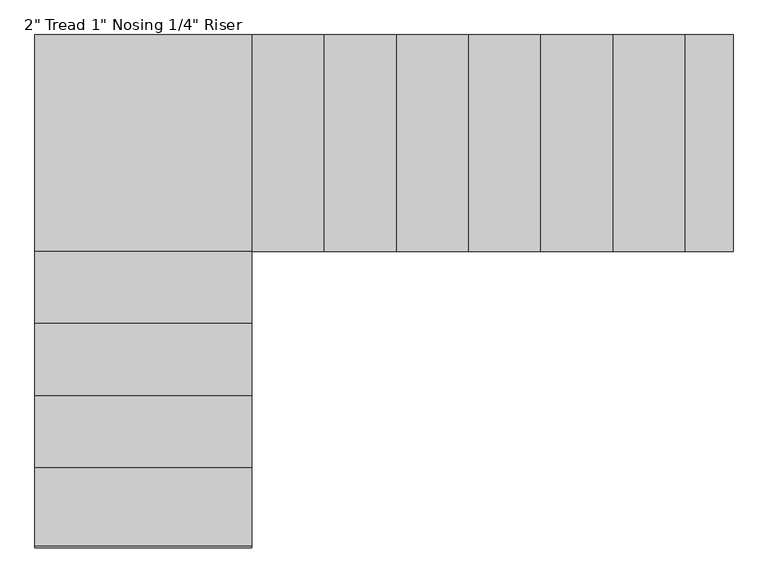
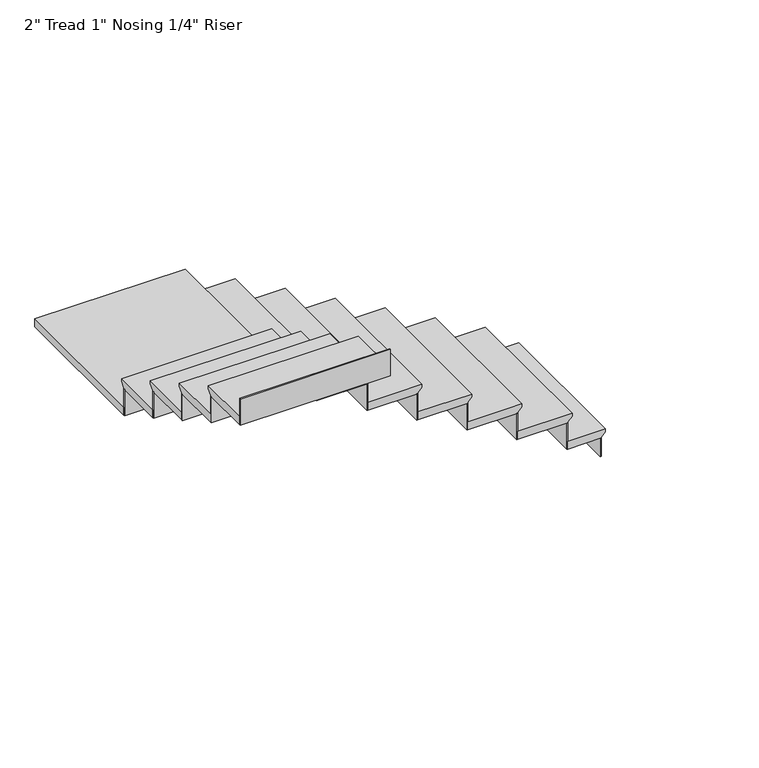
"""IFC4 building model written with IfcOpenShell, lengths in millimetres: stair flight geometry."""

from ifc_helpers import new_model, si_unit, origin, place, context, project, spatial, faceted_brep, source, transform, mapped, element, save


def stair_flight_890a58f3(model_context):
    return source(origin(), model_context, "Body", "Brep", [
        faceted_brep([(-442.4415084, 5282.3381995, 19200.2833333), (-442.4415084, 5282.3381995, 19219.3333333), (-442.4415084, 4368.3146777, 19219.3333333), (-442.4415084, 4368.3146777, 19200.2833333), (-467.8415084, 5282.3381995, 19174.8833333), (-467.8415084, 4368.3146777, 19174.8833333), (-671.0415084, 5282.3381995, 19219.3333333), (-671.0415084, 4368.3146777, 19219.3333333), (-467.8415084, 4368.3146777, 19168.5333333), (-671.0415084, 4368.3146777, 19168.5333333), (-671.0415084, 5282.3381995, 19168.5333333), (-467.8415084, 5282.3381995, 19168.5333333)], [[[0, 1, 2, 3]], [[4, 0, 3, 5]], [[2, 1, 6, 7]], [[8, 9, 10, 11]], [[2, 7, 9, 8, 5, 3]], [[8, 11, 4, 5]], [[6, 1, 0, 4, 11, 10]], [[7, 6, 10, 9]]]),
        faceted_brep([(-467.8415084, 5282.3381995, 19168.5333333), (-467.8415084, 5282.3381995, 19050.0), (-474.1915084, 5282.3381995, 19050.0), (-474.1915084, 5282.3381995, 19168.5333333), (-467.8415084, 4368.3146777, 19168.5333333), (-474.1915084, 4368.3146777, 19168.5333333), (-474.1915084, 4368.3146777, 19050.0), (-467.8415084, 4368.3146777, 19050.0)], [[[0, 1, 2, 3]], [[4, 5, 6, 7]], [[1, 0, 4, 7]], [[2, 1, 7, 6]], [[3, 2, 6, 5]], [[0, 3, 5, 4]]]),
        faceted_brep([(-671.0415084, 5282.3381995, 19337.8666667), (-671.0415084, 5282.3381995, 19168.5333333), (-677.3915084, 5282.3381995, 19168.5333333), (-677.3915084, 5282.3381995, 19337.8666667), (-671.0415084, 4368.3146777, 19337.8666667), (-677.3915084, 4368.3146777, 19337.8666667), (-677.3915084, 4368.3146777, 19168.5333333), (-671.0415084, 4368.3146777, 19168.5333333)], [[[0, 1, 2, 3]], [[4, 5, 6, 7]], [[1, 0, 4, 7]], [[2, 1, 7, 6]], [[3, 2, 6, 5]], [[0, 3, 5, 4]]]),
        faceted_brep([(-645.6415084, 4368.3146777, 19388.6666667), (-645.6415084, 5282.3381995, 19388.6666667), (-975.8415084, 5282.3381995, 19388.6666667), (-975.8415084, 4368.3146777, 19388.6666667), (-671.0415084, 4368.3146777, 19337.8666667), (-975.8415084, 4368.3146777, 19337.8666667), (-975.8415084, 5282.3381995, 19337.8666667), (-671.0415084, 5282.3381995, 19337.8666667), (-671.0415084, 4368.3146777, 19344.2166667), (-645.6415084, 4368.3146777, 19369.6166667), (-671.0415084, 5282.3381995, 19344.2166667), (-645.6415084, 5282.3381995, 19369.6166667)], [[[0, 1, 2, 3]], [[4, 5, 6, 7]], [[0, 3, 5, 4, 8, 9]], [[4, 7, 10, 8]], [[2, 1, 11, 10, 7, 6]], [[3, 2, 6, 5]], [[11, 1, 0, 9]], [[10, 11, 9, 8]]]),
        faceted_brep([(-975.8415084, 5282.3381995, 19507.2), (-975.8415084, 5282.3381995, 19337.8666667), (-982.1915084, 5282.3381995, 19337.8666667), (-982.1915084, 5282.3381995, 19507.2), (-975.8415084, 4368.3146777, 19507.2), (-982.1915084, 4368.3146777, 19507.2), (-982.1915084, 4368.3146777, 19337.8666667), (-975.8415084, 4368.3146777, 19337.8666667)], [[[0, 1, 2, 3]], [[4, 5, 6, 7]], [[1, 0, 4, 7]], [[2, 1, 7, 6]], [[3, 2, 6, 5]], [[0, 3, 5, 4]]]),
        faceted_brep([(-950.4415084, 4368.3146777, 19558.0), (-950.4415084, 5282.3381995, 19558.0), (-1280.6415084, 5282.3381995, 19558.0), (-1280.6415084, 4368.3146777, 19558.0), (-975.8415084, 4368.3146777, 19507.2), (-1280.6415084, 4368.3146777, 19507.2), (-1280.6415084, 5282.3381995, 19507.2), (-975.8415084, 5282.3381995, 19507.2), (-975.8415084, 4368.3146777, 19513.55), (-950.4415084, 4368.3146777, 19538.95), (-975.8415084, 5282.3381995, 19513.55), (-950.4415084, 5282.3381995, 19538.95)], [[[0, 1, 2, 3]], [[4, 5, 6, 7]], [[0, 3, 5, 4, 8, 9]], [[4, 7, 10, 8]], [[2, 1, 11, 10, 7, 6]], [[3, 2, 6, 5]], [[11, 1, 0, 9]], [[10, 11, 9, 8]]]),
        faceted_brep([(-1280.6415084, 5282.3381995, 19676.5333333), (-1280.6415084, 5282.3381995, 19507.2), (-1286.9915084, 5282.3381995, 19507.2), (-1286.9915084, 5282.3381995, 19676.5333333), (-1280.6415084, 4368.3146777, 19676.5333333), (-1286.9915084, 4368.3146777, 19676.5333333), (-1286.9915084, 4368.3146777, 19507.2), (-1280.6415084, 4368.3146777, 19507.2)], [[[0, 1, 2, 3]], [[4, 5, 6, 7]], [[1, 0, 4, 7]], [[2, 1, 7, 6]], [[3, 2, 6, 5]], [[0, 3, 5, 4]]]),
        faceted_brep([(-1255.2415084, 4368.3146777, 19727.3333333), (-1255.2415084, 5282.3381995, 19727.3333333), (-1585.4415084, 5282.3381995, 19727.3333333), (-1585.4415084, 4368.3146777, 19727.3333333), (-1280.6415084, 4368.3146777, 19676.5333333), (-1585.4415084, 4368.3146777, 19676.5333333), (-1585.4415084, 5282.3381995, 19676.5333333), (-1280.6415084, 5282.3381995, 19676.5333333), (-1280.6415084, 4368.3146777, 19682.8833333), (-1255.2415084, 4368.3146777, 19708.2833333), (-1280.6415084, 5282.3381995, 19682.8833333), (-1255.2415084, 5282.3381995, 19708.2833333)], [[[0, 1, 2, 3]], [[4, 5, 6, 7]], [[0, 3, 5, 4, 8, 9]], [[4, 7, 10, 8]], [[2, 1, 11, 10, 7, 6]], [[3, 2, 6, 5]], [[11, 1, 0, 9]], [[10, 11, 9, 8]]]),
        faceted_brep([(-1585.4415084, 5282.3381995, 19845.8666667), (-1585.4415084, 5282.3381995, 19676.5333333), (-1591.7915084, 5282.3381995, 19676.5333333), (-1591.7915084, 5282.3381995, 19845.8666667), (-1585.4415084, 4368.3146777, 19845.8666667), (-1591.7915084, 4368.3146777, 19845.8666667), (-1591.7915084, 4368.3146777, 19676.5333333), (-1585.4415084, 4368.3146777, 19676.5333333)], [[[0, 1, 2, 3]], [[4, 5, 6, 7]], [[1, 0, 4, 7]], [[2, 1, 7, 6]], [[3, 2, 6, 5]], [[0, 3, 5, 4]]]),
        faceted_brep([(-1560.0415084, 4368.3146777, 19896.6666667), (-1560.0415084, 5282.3381995, 19896.6666667), (-1890.2415084, 5282.3381995, 19896.6666667), (-1890.2415084, 4368.3146777, 19896.6666667), (-1585.4415084, 4368.3146777, 19845.8666667), (-1890.2415084, 4368.3146777, 19845.8666667), (-1890.2415084, 5282.3381995, 19845.8666667), (-1585.4415084, 5282.3381995, 19845.8666667), (-1585.4415084, 4368.3146777, 19852.2166667), (-1560.0415084, 4368.3146777, 19877.6166667), (-1585.4415084, 5282.3381995, 19852.2166667), (-1560.0415084, 5282.3381995, 19877.6166667)], [[[0, 1, 2, 3]], [[4, 5, 6, 7]], [[0, 3, 5, 4, 8, 9]], [[4, 7, 10, 8]], [[2, 1, 11, 10, 7, 6]], [[3, 2, 6, 5]], [[11, 1, 0, 9]], [[10, 11, 9, 8]]]),
        faceted_brep([(-1890.2415084, 5282.3381995, 20015.2), (-1890.2415084, 5282.3381995, 19845.8666667), (-1896.5915084, 5282.3381995, 19845.8666667), (-1896.5915084, 5282.3381995, 20015.2), (-1890.2415084, 4368.3146777, 20015.2), (-1896.5915084, 4368.3146777, 20015.2), (-1896.5915084, 4368.3146777, 19845.8666667), (-1890.2415084, 4368.3146777, 19845.8666667)], [[[0, 1, 2, 3]], [[4, 5, 6, 7]], [[1, 0, 4, 7]], [[2, 1, 7, 6]], [[3, 2, 6, 5]], [[0, 3, 5, 4]]]),
        faceted_brep([(-1864.8415084, 4368.3146777, 20066.0), (-1864.8415084, 5282.3381995, 20066.0), (-2195.0415084, 5282.3381995, 20066.0), (-2195.0415084, 4368.3146777, 20066.0), (-1890.2415084, 4368.3146777, 20015.2), (-2195.0415084, 4368.3146777, 20015.2), (-2195.0415084, 5282.3381995, 20015.2), (-1890.2415084, 5282.3381995, 20015.2), (-1890.2415084, 4368.3146777, 20021.55), (-1864.8415084, 4368.3146777, 20046.95), (-1890.2415084, 5282.3381995, 20021.55), (-1864.8415084, 5282.3381995, 20046.95)], [[[0, 1, 2, 3]], [[4, 5, 6, 7]], [[0, 3, 5, 4, 8, 9]], [[4, 7, 10, 8]], [[2, 1, 11, 10, 7, 6]], [[3, 2, 6, 5]], [[11, 1, 0, 9]], [[10, 11, 9, 8]]]),
        faceted_brep([(-2195.0415084, 5282.3381995, 20184.5333333), (-2195.0415084, 5282.3381995, 20015.2), (-2201.3915084, 5282.3381995, 20015.2), (-2201.3915084, 5282.3381995, 20184.5333333), (-2195.0415084, 4368.3146777, 20184.5333333), (-2201.3915084, 4368.3146777, 20184.5333333), (-2201.3915084, 4368.3146777, 20015.2), (-2195.0415084, 4368.3146777, 20015.2)], [[[0, 1, 2, 3]], [[4, 5, 6, 7]], [[1, 0, 4, 7]], [[2, 1, 7, 6]], [[3, 2, 6, 5]], [[0, 3, 5, 4]]]),
        faceted_brep([(-2169.6415084, 4368.3146777, 20235.3333333), (-2169.6415084, 5282.3381995, 20235.3333333), (-2499.8415084, 5282.3381995, 20235.3333333), (-2499.8415084, 4368.3146777, 20235.3333333), (-2195.0415084, 4368.3146777, 20184.5333333), (-2499.8415084, 4368.3146777, 20184.5333333), (-2499.8415084, 5282.3381995, 20184.5333333), (-2195.0415084, 5282.3381995, 20184.5333333), (-2195.0415084, 4368.3146777, 20190.8833333), (-2169.6415084, 4368.3146777, 20216.2833333), (-2195.0415084, 5282.3381995, 20190.8833333), (-2169.6415084, 5282.3381995, 20216.2833333)], [[[0, 1, 2, 3]], [[4, 5, 6, 7]], [[0, 3, 5, 4, 8, 9]], [[4, 7, 10, 8]], [[2, 1, 11, 10, 7, 6]], [[3, 2, 6, 5]], [[11, 1, 0, 9]], [[10, 11, 9, 8]]]),
        faceted_brep([(-2499.8415084, 5282.3381995, 20353.8666667), (-2499.8415084, 5282.3381995, 20184.5333333), (-2506.1915084, 5282.3381995, 20184.5333333), (-2506.1915084, 5282.3381995, 20353.8666667), (-2499.8415084, 4368.3146777, 20353.8666667), (-2506.1915084, 4368.3146777, 20353.8666667), (-2506.1915084, 4368.3146777, 20184.5333333), (-2499.8415084, 4368.3146777, 20184.5333333)], [[[0, 1, 2, 3]], [[4, 5, 6, 7]], [[1, 0, 4, 7]], [[2, 1, 7, 6]], [[3, 2, 6, 5]], [[0, 3, 5, 4]]]),
        faceted_brep([(-3388.8415084, 5282.3381995, 20404.6666667), (-3388.8415084, 4342.9146777, 20404.6666667), (-2474.4415084, 4342.9146777, 20404.6666667), (-2474.4415084, 5282.3381995, 20404.6666667), (-2474.4415084, 4368.3146777, 20353.8666667), (-2474.4415084, 4342.9146777, 20353.8666667), (-3388.8415084, 4342.9146777, 20353.8666667), (-3388.8415084, 5282.3381995, 20353.8666667), (-2499.8415084, 5282.3381995, 20353.8666667), (-2499.8415084, 4368.3146777, 20353.8666667), (-2474.4415084, 4368.3146777, 20385.6166667), (-2474.4415084, 5282.3381995, 20385.6166667), (-2499.8415084, 4368.3146777, 20360.2166667), (-2499.8415084, 5282.3381995, 20360.2166667)], [[[0, 1, 2, 3]], [[4, 5, 6, 7, 8, 9]], [[3, 2, 5, 4, 10, 11]], [[4, 9, 12, 10]], [[9, 8, 13, 12]], [[0, 3, 11, 13, 8, 7]], [[1, 0, 7, 6]], [[2, 1, 6, 5]], [[13, 11, 10, 12]]]),
        faceted_brep([(-3388.8415084, 4342.9146777, 20523.2), (-3388.8415084, 4342.9146777, 20353.8666667), (-3388.8415084, 4336.5646777, 20353.8666667), (-3388.8415084, 4336.5646777, 20523.2), (-2474.4415084, 4342.9146777, 20523.2), (-2474.4415084, 4336.5646777, 20523.2), (-2474.4415084, 4336.5646777, 20353.8666667), (-2474.4415084, 4342.9146777, 20353.8666667)], [[[0, 1, 2, 3]], [[4, 5, 6, 7]], [[1, 0, 4, 7]], [[2, 1, 7, 6]], [[3, 2, 6, 5]], [[0, 3, 5, 4]]]),
        faceted_brep([(-2474.4415084, 4368.3146777, 20574.0), (-3388.8415084, 4368.3146777, 20574.0), (-3388.8415084, 4037.7382512, 20574.0), (-2474.4415084, 4037.7382512, 20574.0), (-2474.4415084, 4342.9146777, 20523.2), (-2474.4415084, 4037.7382512, 20523.2), (-3388.8415084, 4037.7382512, 20523.2), (-3388.8415084, 4342.9146777, 20523.2), (-2474.4415084, 4342.9146777, 20529.55), (-2474.4415084, 4368.3146777, 20554.95), (-3388.8415084, 4342.9146777, 20529.55), (-3388.8415084, 4368.3146777, 20554.95)], [[[0, 1, 2, 3]], [[4, 5, 6, 7]], [[0, 3, 5, 4, 8, 9]], [[4, 7, 10, 8]], [[2, 1, 11, 10, 7, 6]], [[3, 2, 6, 5]], [[11, 1, 0, 9]], [[10, 11, 9, 8]]]),
        faceted_brep([(-3388.8415084, 4037.7382512, 20692.5333333), (-3388.8415084, 4037.7382512, 20523.2), (-3388.8415084, 4031.3882512, 20523.2), (-3388.8415084, 4031.3882512, 20692.5333333), (-2474.4415084, 4037.7382512, 20692.5333333), (-2474.4415084, 4031.3882512, 20692.5333333), (-2474.4415084, 4031.3882512, 20523.2), (-2474.4415084, 4037.7382512, 20523.2)], [[[0, 1, 2, 3]], [[4, 5, 6, 7]], [[1, 0, 4, 7]], [[2, 1, 7, 6]], [[3, 2, 6, 5]], [[0, 3, 5, 4]]]),
        faceted_brep([(-2474.4415084, 4063.1382512, 20743.3333333), (-3388.8415084, 4063.1382512, 20743.3333333), (-3388.8415084, 3732.938277, 20743.3333333), (-2474.4415084, 3732.938277, 20743.3333333), (-2474.4415084, 4037.7382512, 20692.5333333), (-2474.4415084, 3732.938277, 20692.5333333), (-3388.8415084, 3732.938277, 20692.5333333), (-3388.8415084, 4037.7382512, 20692.5333333), (-2474.4415084, 4037.7382512, 20698.8833333), (-2474.4415084, 4063.1382512, 20724.2833333), (-3388.8415084, 4037.7382512, 20698.8833333), (-3388.8415084, 4063.1382512, 20724.2833333)], [[[0, 1, 2, 3]], [[4, 5, 6, 7]], [[0, 3, 5, 4, 8, 9]], [[4, 7, 10, 8]], [[2, 1, 11, 10, 7, 6]], [[3, 2, 6, 5]], [[11, 1, 0, 9]], [[10, 11, 9, 8]]]),
        faceted_brep([(-3388.8415084, 3732.938277, 20861.8666667), (-3388.8415084, 3732.938277, 20692.5333333), (-3388.8415084, 3726.588277, 20692.5333333), (-3388.8415084, 3726.588277, 20861.8666667), (-2474.4415084, 3732.938277, 20861.8666667), (-2474.4415084, 3726.588277, 20861.8666667), (-2474.4415084, 3726.588277, 20692.5333333), (-2474.4415084, 3732.938277, 20692.5333333)], [[[0, 1, 2, 3]], [[4, 5, 6, 7]], [[1, 0, 4, 7]], [[2, 1, 7, 6]], [[3, 2, 6, 5]], [[0, 3, 5, 4]]]),
        faceted_brep([(-2474.4415084, 3758.338277, 20912.6666667), (-3388.8415084, 3758.338277, 20912.6666667), (-3388.8415084, 3428.1383028, 20912.6666667), (-2474.4415084, 3428.1383028, 20912.6666667), (-2474.4415084, 3732.938277, 20861.8666667), (-2474.4415084, 3428.1383028, 20861.8666667), (-3388.8415084, 3428.1383028, 20861.8666667), (-3388.8415084, 3732.938277, 20861.8666667), (-2474.4415084, 3732.938277, 20868.2166667), (-2474.4415084, 3758.338277, 20893.6166667), (-3388.8415084, 3732.938277, 20868.2166667), (-3388.8415084, 3758.338277, 20893.6166667)], [[[0, 1, 2, 3]], [[4, 5, 6, 7]], [[0, 3, 5, 4, 8, 9]], [[4, 7, 10, 8]], [[2, 1, 11, 10, 7, 6]], [[3, 2, 6, 5]], [[11, 1, 0, 9]], [[10, 11, 9, 8]]]),
        faceted_brep([(-3388.8415084, 3428.1383028, 21031.2), (-3388.8415084, 3428.1383028, 20861.8666667), (-3388.8415084, 3421.7883028, 20861.8666667), (-3388.8415084, 3421.7883028, 21031.2), (-2474.4415084, 3428.1383028, 21031.2), (-2474.4415084, 3421.7883028, 21031.2), (-2474.4415084, 3421.7883028, 20861.8666667), (-2474.4415084, 3428.1383028, 20861.8666667)], [[[0, 1, 2, 3]], [[4, 5, 6, 7]], [[1, 0, 4, 7]], [[2, 1, 7, 6]], [[3, 2, 6, 5]], [[0, 3, 5, 4]]]),
        faceted_brep([(-3388.8415084, 3123.3383287, 21200.5333333), (-3388.8415084, 3123.3383287, 21031.2), (-3388.8415084, 3116.9883287, 21031.2), (-3388.8415084, 3116.9883287, 21200.5333333), (-2474.4415084, 3123.3383287, 21200.5333333), (-2474.4415084, 3116.9883287, 21200.5333333), (-2474.4415084, 3116.9883287, 21031.2), (-2474.4415084, 3123.3383287, 21031.2)], [[[0, 1, 2, 3]], [[4, 5, 6, 7]], [[1, 0, 4, 7]], [[2, 1, 7, 6]], [[3, 2, 6, 5]], [[0, 3, 5, 4]]]),
        faceted_brep([(-2474.4415084, 3453.5383028, 21082.0), (-3388.8415084, 3453.5383028, 21082.0), (-3388.8415084, 3123.3383287, 21082.0), (-2474.4415084, 3123.3383287, 21082.0), (-2474.4415084, 3428.1383028, 21031.2), (-2474.4415084, 3123.3383287, 21031.2), (-3388.8415084, 3123.3383287, 21031.2), (-3388.8415084, 3428.1383028, 21031.2), (-2474.4415084, 3428.1383028, 21037.55), (-2474.4415084, 3453.5383028, 21062.95), (-3388.8415084, 3428.1383028, 21037.55), (-3388.8415084, 3453.5383028, 21062.95)], [[[0, 1, 2, 3]], [[4, 5, 6, 7]], [[0, 3, 5, 4, 8, 9]], [[4, 7, 10, 8]], [[2, 1, 11, 10, 7, 6]], [[3, 2, 6, 5]], [[11, 1, 0, 9]], [[10, 11, 9, 8]]]),
    ])


if __name__ == "__main__":
    model = new_model("IFC4")
    model_context = context("Model", 3, world=origin())
    ifc_project = project(units=[si_unit("LENGTHUNIT", "METRE", prefix="MILLI")], contexts=[model_context])
    site = spatial("IfcSite", under=ifc_project)
    building = spatial("IfcBuilding", under=site)
    placement = place(None, origin())
    stair_flight_shape = stair_flight_890a58f3(model_context)
    element("IfcStairFlight", 1, ObjectType="2\" Tread 1\" Nosing 1/4\" Riser", at=placement, inside=building, context=model_context, shape_type="MappedRepresentation", body=[
        mapped(stair_flight_shape, transform((0.0, 0.0, 0.0), x_axis=(1.0, 0.0, 0.0), y_axis=(0.0, 1.0, 0.0), z_axis=(0.0, 0.0, 1.0))),
    ])
    save(model, "model.ifc")
